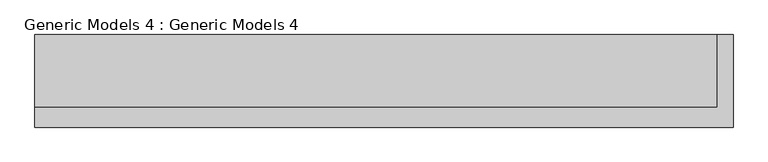
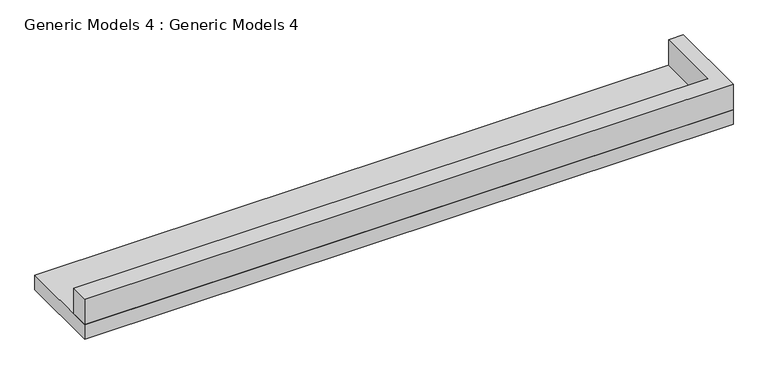
"""IFC4 building model written with IfcOpenShell, lengths in millimetres: proxy geometry, Generic Models 4 : Generic Models 4."""

from ifc_helpers import new_model, si_unit, frame, origin, place, context, project, spatial, polyline, outline, extrude, source, transform, mapped, element, save


def generic_models_4_generic_models_4_9f1effd6(model_context):
    return source(origin(), model_context, "Body", "SweptSolid", [
        extrude(outline(polyline([(-16217.2212454, -15454.2906536), (-16217.2212454, -15171.132201), (-6500.8195233, -15171.132201), (-6500.8195233, -14134.7752569), (-6272.2195233, -14134.7752569), (-6272.2195233, -15454.2906536), (-16217.2212454, -15454.2906536)])), frame((0.0, 0.0, 3588.5355704), z_axis=(0.0, 0.0, 1.0), x_axis=(1.0, 0.0, 0.0)), (0.0, 0.0, 1.0), 413.2660792),
        extrude(outline(polyline([(-6272.2195233, -15454.2906536), (-16217.2212454, -15454.2906536), (-16217.2212454, -14134.7752569), (-6272.2195233, -14134.7752569), (-6272.2195233, -15454.2906536)])), frame((0.0, 0.0, 3352.8), z_axis=(0.0, 0.0, 1.0), x_axis=(1.0, 0.0, 0.0)), (0.0, 0.0, 1.0), 235.7355704),
    ])


if __name__ == "__main__":
    model = new_model("IFC4")
    model_context = context("Model", 3, world=origin())
    ifc_project = project(units=[si_unit("LENGTHUNIT", "METRE", prefix="MILLI")], contexts=[model_context])
    site = spatial("IfcSite", under=ifc_project)
    building = spatial("IfcBuilding", under=site)
    placement = place(None, origin())
    generic_models_4_generic_models_4_shape = generic_models_4_generic_models_4_9f1effd6(model_context)
    element("IfcBuildingElementProxy", 1, Name="Generic Models 4 : Generic Models 4", ObjectType="Generic Models 4 : Generic Models 4", at=placement, inside=building, context=model_context, shape_type="MappedRepresentation", body=[
        mapped(generic_models_4_generic_models_4_shape, transform((0.0, 0.0, 0.0), x_axis=(1.0, 0.0, 0.0), y_axis=(0.0, 1.0, 0.0), z_axis=(0.0, 0.0, 1.0))),
    ])
    save(model, "model.ifc")
